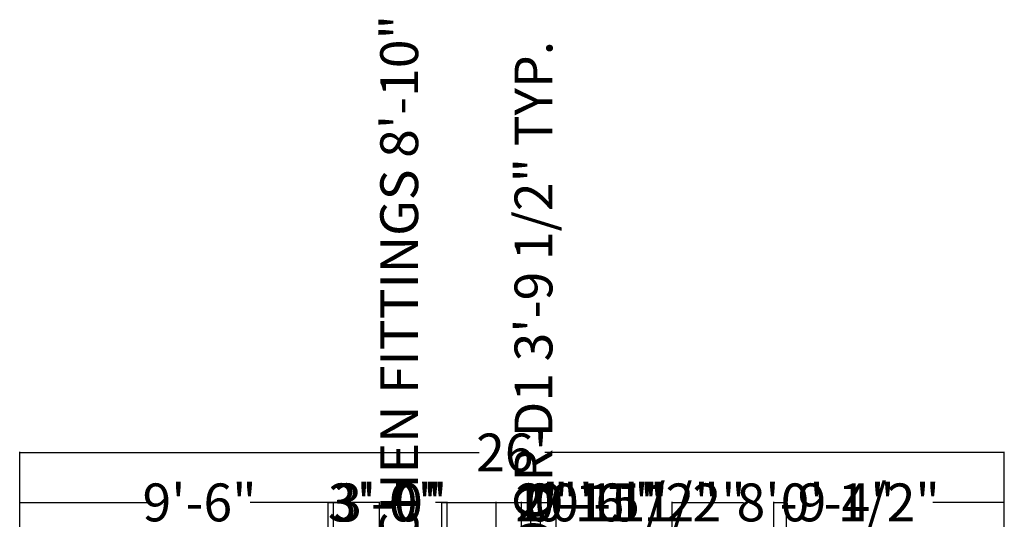
# Model space of a CAD drawing. Units: inches. Extents: x -51 to 1118, y -44 to 791.
# Tile 6 of 8: x 28 to 340, y 633 to 791. Entities that reach past the tile are written whole.
import ezdxf

# ---------------------------------------------------------------- set-up
doc = ezdxf.new("R2010")
doc.units = ezdxf.units.IN
doc.header["$MEASUREMENT"] = 0
doc.layers.add('A-ANNO-DIMS', color=2, linetype='Continuous', lineweight=18)
doc.styles.get("Standard").update_dxf_attribs({"font": 'arial.ttf'})
doc.dimstyles.get("Standard").update_dxf_attribs({"dimtxt": 12, "dimasz": 0.18, "dimexe": 0.18, "dimexo": 0.0625, "dimgap": 0.09, "dimtad": 0, "dimdec": 1, "dimzin": 0, "dimdsep": 46, "dimlunit": 3, "dimtxsty": 'Standard', "dimcen": 0.09, "dimadec": 0, "dimazin": 0, "dimtfac": 1, "dimtdec": 1, "dimtofl": 0, "dimtmove": 0, "dimatfit": 3, "dimfxl": 1, "dimtolj": 1, "dimtzin": 0, "dimarcsym": 0})

# ---------------------------------------------------------------- blocks, each defined once
blk = doc.blocks.new('*D10')
at = {"layer": 'A-ANNO-DIMS', "color": 0, "lineweight": -2, "transparency": 16777216}
for p, q in [((28.02, 606), (28.02, 654.38)), ((28.2, 654.2), (173.65, 654.2)), ((339.84, 654.2), (194.4, 654.2)), ((340.02, 606), (340.02, 654.38))]:
    blk.add_line(p, q, dxfattribs=at)
at = {"layer": 'A-ANNO-DIMS', "color": 0, "transparency": 16777216}
for points in [[(28.2, 654.23), (28.2, 654.17), (28.02, 654.2)], [(339.84, 654.23), (339.84, 654.17), (340.02, 654.2)]]:
    blk.add_solid(points, dxfattribs=at)
at = {"layer": 'Defpoints', "color": 0, "transparency": 16777216}
for p in [(340.02, 654.2), (28.02, 605.94), (340.02, 605.94)]:
    blk.add_point(p, dxfattribs=at)
at = {"layer": 'A-ANNO-DIMS', "color": 0, "transparency": 16777216, "insert": (184.02, 654.2), "char_height": 12, "attachment_point": 5}
blk.add_mtext("\\A1;26'", dxfattribs=at)
blk = doc.blocks.new('*D20')
at = {"layer": 'A-ANNO-DIMS', "color": 0, "lineweight": -2, "transparency": 16777216}
for p, q in [((184.08, 605.94), (191.01, 605.94)), ((190.83, 605.94), (190.83, 606.12)), ((190.83, 560.7), (190.83, 605.76)), ((184.08, 560.52), (191.01, 560.52))]:
    blk.add_line(p, q, dxfattribs=at)
at = {"layer": 'A-ANNO-DIMS', "color": 0, "transparency": 16777216}
for points in [[(190.8, 605.76), (190.86, 605.76), (190.83, 605.94)], [(190.8, 560.7), (190.86, 560.7), (190.83, 560.52)]]:
    blk.add_solid(points, dxfattribs=at)
at = {"layer": 'Defpoints', "color": 0, "transparency": 16777216}
for p in [(184.02, 605.94), (190.83, 605.94), (184.02, 560.52)]:
    blk.add_point(p, dxfattribs=at)
at = {"layer": 'A-ANNO-DIMS', "color": 0, "transparency": 16777216, "insert": (190.83, 696.98), "char_height": 12, "attachment_point": 5, "rotation": 90}
blk.add_mtext('\\A1;DOOR D1 3\'-9 1/2" TYP.', dxfattribs=at)
blk = doc.blocks.new('*D34')
at = {"layer": 'A-ANNO-DIMS', "color": 0, "lineweight": -2, "transparency": 16777216}
for p, q in [((132.45, 596.14), (148.46, 596.14)), ((148.28, 596.14), (148.28, 596.32)), ((148.28, 490.32), (148.28, 595.96)), ((132.45, 490.14), (148.46, 490.14))]:
    blk.add_line(p, q, dxfattribs=at)
at = {"layer": 'A-ANNO-DIMS', "color": 0, "transparency": 16777216}
for points in [[(148.25, 595.96), (148.31, 595.96), (148.28, 596.14)], [(148.25, 490.32), (148.31, 490.32), (148.28, 490.14)]]:
    blk.add_solid(points, dxfattribs=at)
at = {"layer": 'Defpoints', "color": 0, "transparency": 16777216}
for p in [(132.38, 596.14), (148.28, 596.14), (132.38, 490.14)]:
    blk.add_point(p, dxfattribs=at)
at = {"layer": 'A-ANNO-DIMS', "color": 0, "transparency": 16777216, "insert": (148.28, 696.39), "char_height": 12, "attachment_point": 5, "rotation": 90}
blk.add_mtext('\\A1;KITCHEN FITTINGS 8\'-10"', dxfattribs=at)
blk = doc.blocks.new('*D43')
at = {"layer": 'A-ANNO-DIMS', "color": 0, "lineweight": -2, "transparency": 16777216}
for p, q in [((187.02, 597), (187.02, 638.57)), ((187.2, 638.39), (192.84, 638.39)), ((193.02, 597), (193.02, 638.57)), ((193.02, 638.39), (193.2, 638.39))]:
    blk.add_line(p, q, dxfattribs=at)
at = {"layer": 'A-ANNO-DIMS', "color": 0, "transparency": 16777216}
for points in [[(187.2, 638.42), (187.2, 638.36), (187.02, 638.39)], [(192.84, 638.42), (192.84, 638.36), (193.02, 638.39)]]:
    blk.add_solid(points, dxfattribs=at)
at = {"layer": 'Defpoints', "color": 0, "transparency": 16777216}
for p in [(193.02, 638.39), (187.02, 596.94), (193.02, 596.94)]:
    blk.add_point(p, dxfattribs=at)
at = {"layer": 'A-ANNO-DIMS', "color": 0, "transparency": 16777216, "insert": (209.24, 638.39), "char_height": 12, "attachment_point": 5}
blk.add_mtext('\\A1;0\'-6"', dxfattribs=at)
blk = doc.blocks.new('*D48')
at = {"layer": 'A-ANNO-DIMS', "color": 0, "lineweight": -2, "transparency": 16777216}
for p, q in [((28.02, 606), (28.02, 638.57)), ((28.2, 638.39), (68.98, 638.39)), ((141.84, 638.39), (101.06, 638.39)), ((142.02, 606), (142.02, 638.57))]:
    blk.add_line(p, q, dxfattribs=at)
at = {"layer": 'A-ANNO-DIMS', "color": 0, "transparency": 16777216}
for points in [[(28.2, 638.42), (28.2, 638.36), (28.02, 638.39)], [(141.84, 638.42), (141.84, 638.36), (142.02, 638.39)]]:
    blk.add_solid(points, dxfattribs=at)
at = {"layer": 'Defpoints', "color": 0, "transparency": 16777216}
for p in [(142.02, 638.39), (28.02, 605.94), (142.02, 605.94)]:
    blk.add_point(p, dxfattribs=at)
at = {"layer": 'A-ANNO-DIMS', "color": 0, "transparency": 16777216, "insert": (85.02, 638.39), "char_height": 12, "attachment_point": 5}
blk.add_mtext('\\A1;9\'-6"', dxfattribs=at)
blk = doc.blocks.new('*D49')
at = {"layer": 'A-ANNO-DIMS', "color": 0, "lineweight": -2, "transparency": 16777216}
for p, q in [((234.77, 606), (234.77, 638.57)), ((234.95, 638.39), (257.37, 638.39)), ((339.84, 638.39), (317.42, 638.39)), ((340.02, 606), (340.02, 638.57))]:
    blk.add_line(p, q, dxfattribs=at)
at = {"layer": 'A-ANNO-DIMS', "color": 0, "transparency": 16777216}
for points in [[(234.95, 638.42), (234.95, 638.36), (234.77, 638.39)], [(339.84, 638.42), (339.84, 638.36), (340.02, 638.39)]]:
    blk.add_solid(points, dxfattribs=at)
at = {"layer": 'Defpoints', "color": 0, "transparency": 16777216}
for p in [(340.02, 638.39), (234.77, 605.94), (340.02, 605.94)]:
    blk.add_point(p, dxfattribs=at)
at = {"layer": 'A-ANNO-DIMS', "color": 0, "transparency": 16777216, "insert": (287.4, 638.39), "char_height": 12, "attachment_point": 5}
blk.add_mtext('\\A1;8\'-9 1/2"', dxfattribs=at)
blk = doc.blocks.new('*D55')
at = {"layer": 'A-ANNO-DIMS', "color": 0, "lineweight": -2, "transparency": 16777216}
for p, q in [((193.02, 108), (193.02, 638.57)), ((193.2, 638.39), (197.79, 638.39)), ((197.97, 108), (197.97, 638.57)), ((197.97, 638.39), (198.15, 638.39))]:
    blk.add_line(p, q, dxfattribs=at)
at = {"layer": 'A-ANNO-DIMS', "color": 0, "transparency": 16777216}
for points in [[(193.2, 638.42), (193.2, 638.36), (193.02, 638.39)], [(197.79, 638.42), (197.79, 638.36), (197.97, 638.39)]]:
    blk.add_solid(points, dxfattribs=at)
at = {"layer": 'Defpoints', "color": 0, "transparency": 16777216}
for p in [(197.97, 638.39), (193.02, 107.94), (197.97, 107.94)]:
    blk.add_point(p, dxfattribs=at)
at = {"layer": 'A-ANNO-DIMS', "color": 0, "transparency": 16777216, "insert": (214.19, 638.39), "char_height": 12, "attachment_point": 5}
blk.add_mtext('\\A1;0\'-5"', dxfattribs=at)
blk = doc.blocks.new('*D57')
at = {"layer": 'A-ANNO-DIMS', "color": 0, "lineweight": -2, "transparency": 16777216}
for p, q in [((179.02, 57), (179.02, 638.57)), ((179.2, 638.39), (189.84, 638.39)), ((190.02, 57), (190.02, 638.57)), ((190.02, 638.39), (190.2, 638.39))]:
    blk.add_line(p, q, dxfattribs=at)
at = {"layer": 'A-ANNO-DIMS', "color": 0, "transparency": 16777216}
for points in [[(179.2, 638.42), (179.2, 638.36), (179.02, 638.39)], [(189.84, 638.42), (189.84, 638.36), (190.02, 638.39)]]:
    blk.add_solid(points, dxfattribs=at)
at = {"layer": 'Defpoints', "color": 0, "transparency": 16777216}
for p in [(190.02, 638.39), (179.02, 56.94), (190.02, 56.94)]:
    blk.add_point(p, dxfattribs=at)
at = {"layer": 'A-ANNO-DIMS', "color": 0, "transparency": 16777216, "insert": (210.9, 638.39), "char_height": 12, "attachment_point": 5}
blk.add_mtext('\\A1;0\'-11"', dxfattribs=at)
blk = doc.blocks.new('*D61')
at = {"layer": 'A-ANNO-DIMS', "color": 0, "lineweight": -2, "transparency": 16777216}
for p, q in [((125.75, 324), (125.75, 638.57)), ((125.93, 638.39), (127.71, 638.39)), ((161.57, 638.39), (159.79, 638.39)), ((161.75, 324), (161.75, 638.57))]:
    blk.add_line(p, q, dxfattribs=at)
at = {"layer": 'A-ANNO-DIMS', "color": 0, "transparency": 16777216}
for points in [[(125.93, 638.42), (125.93, 638.36), (125.75, 638.39)], [(161.57, 638.42), (161.57, 638.36), (161.75, 638.39)]]:
    blk.add_solid(points, dxfattribs=at)
at = {"layer": 'Defpoints', "color": 0, "transparency": 16777216}
for p in [(161.75, 638.39), (125.75, 323.94), (161.75, 323.94)]:
    blk.add_point(p, dxfattribs=at)
at = {"layer": 'A-ANNO-DIMS', "color": 0, "transparency": 16777216, "insert": (143.75, 638.39), "char_height": 12, "attachment_point": 5}
blk.add_mtext('\\A1;3\'-0"', dxfattribs=at)
blk = doc.blocks.new('*D62')
at = {"layer": 'A-ANNO-DIMS', "color": 0, "lineweight": -2, "transparency": 16777216}
for p, q in [((161.75, 324), (161.75, 638.57)), ((161.93, 638.39), (186.84, 638.39)), ((187.02, 327), (187.02, 638.57)), ((187.02, 638.39), (187.2, 638.39))]:
    blk.add_line(p, q, dxfattribs=at)
at = {"layer": 'A-ANNO-DIMS', "color": 0, "transparency": 16777216}
for points in [[(161.93, 638.42), (161.93, 638.36), (161.75, 638.39)], [(186.84, 638.42), (186.84, 638.36), (187.02, 638.39)]]:
    blk.add_solid(points, dxfattribs=at)
at = {"layer": 'Defpoints', "color": 0, "transparency": 16777216}
for p in [(187.02, 638.39), (187.02, 326.94), (161.75, 323.94)]:
    blk.add_point(p, dxfattribs=at)
at = {"layer": 'A-ANNO-DIMS', "color": 0, "transparency": 16777216, "insert": (217.32, 638.39), "char_height": 12, "attachment_point": 5}
blk.add_mtext('\\A1;2\'-1 1/2"', dxfattribs=at)
blk = doc.blocks.new('*D63')
at = {"layer": 'A-ANNO-DIMS', "color": 0, "lineweight": -2, "transparency": 16777216}
for p, q in [((127.45, 453), (127.45, 638.57)), ((127.63, 638.39), (129.41, 638.39)), ((163.27, 638.39), (161.48, 638.39)), ((163.45, 453), (163.45, 638.57))]:
    blk.add_line(p, q, dxfattribs=at)
at = {"layer": 'A-ANNO-DIMS', "color": 0, "transparency": 16777216}
for points in [[(127.63, 638.42), (127.63, 638.36), (127.45, 638.39)], [(163.27, 638.42), (163.27, 638.36), (163.45, 638.39)]]:
    blk.add_solid(points, dxfattribs=at)
at = {"layer": 'Defpoints', "color": 0, "transparency": 16777216}
for p in [(163.45, 638.39), (127.45, 452.94), (163.45, 452.94)]:
    blk.add_point(p, dxfattribs=at)
at = {"layer": 'A-ANNO-DIMS', "color": 0, "transparency": 16777216, "insert": (145.45, 638.39), "char_height": 12, "attachment_point": 5}
blk.add_mtext('\\A1;3\'-0"', dxfattribs=at)
blk = doc.blocks.new('*D64')
at = {"layer": 'A-ANNO-DIMS', "color": 0, "lineweight": -2, "transparency": 16777216}
for p, q in [((163.45, 453), (163.45, 638.57)), ((163.63, 638.39), (186.84, 638.39)), ((187.02, 453), (187.02, 638.57)), ((187.02, 638.39), (187.2, 638.39))]:
    blk.add_line(p, q, dxfattribs=at)
at = {"layer": 'A-ANNO-DIMS', "color": 0, "transparency": 16777216}
for points in [[(163.63, 638.42), (163.63, 638.36), (163.45, 638.39)], [(186.84, 638.42), (186.84, 638.36), (187.02, 638.39)]]:
    blk.add_solid(points, dxfattribs=at)
at = {"layer": 'Defpoints', "color": 0, "transparency": 16777216}
for p in [(187.02, 638.39), (163.45, 452.94), (187.02, 452.94)]:
    blk.add_point(p, dxfattribs=at)
at = {"layer": 'A-ANNO-DIMS', "color": 0, "transparency": 16777216, "insert": (221.32, 638.39), "char_height": 12, "attachment_point": 5}
blk.add_mtext('\\A1;1\'-11 1/2"', dxfattribs=at)
blk = doc.blocks.new('*D65')
at = {"layer": 'A-ANNO-DIMS', "color": 0, "lineweight": -2, "transparency": 16777216}
for p, q in [((267.02, 366), (267.02, 638.57)), ((267.2, 638.39), (270.84, 638.39)), ((271.02, 366), (271.02, 638.57)), ((271.02, 638.39), (271.2, 638.39))]:
    blk.add_line(p, q, dxfattribs=at)
at = {"layer": 'A-ANNO-DIMS', "color": 0, "transparency": 16777216}
for points in [[(267.2, 638.42), (267.2, 638.36), (267.02, 638.39)], [(270.84, 638.42), (270.84, 638.36), (271.02, 638.39)]]:
    blk.add_solid(points, dxfattribs=at)
at = {"layer": 'Defpoints', "color": 0, "transparency": 16777216}
for p in [(271.02, 638.39), (267.02, 365.94), (271.02, 365.94)]:
    blk.add_point(p, dxfattribs=at)
at = {"layer": 'A-ANNO-DIMS', "color": 0, "transparency": 16777216, "insert": (287.24, 638.39), "char_height": 12, "attachment_point": 5}
blk.add_mtext('\\A1;0\'-4"', dxfattribs=at)

msp = doc.modelspace()

# ---------------------------------------------------------------- dimensions: what is measured, and where the dimension line sits
at = {"layer": 'A-ANNO-DIMS'}
for base, p1, p2, text, picture, middle in [((148.28, 596.14), (132.38, 490.14), (132.38, 596.14), 'KITCHEN FITTINGS <>', '*D34', (148.28, 696.39)), ((190.83, 605.94), (184.02, 560.52), (184.02, 605.94), 'DOOR D1 <> TYP.', '*D20', (190.83, 696.98))]:
    dim = msp.add_linear_dim(base=base, p1=p1, p2=p2, angle=90, text=text, dimstyle='Standard', override={"dimdec": 1, "dimlfac": 1, "dimrnd": 0, "dimzin": 1, "dimdsep": 46, "dimlunit": 4, "dimfrac": 2}, dxfattribs=at)
    dim.commit()
    dim.dimension.update_dxf_attribs({"geometry": picture, "text_midpoint": middle})
for base, p1, p2, override, picture, middle in [((340.02, 654.2), (28.02, 605.94), (340.02, 605.94), {"dimclrd": 0, "dimclre": 0, "dimclrt": 0}, '*D10', (184.02, 654.2)), ((187.02, 638.39), (161.75, 323.94), (187.02, 326.94), {"dimdec": 1, "dimlfac": 1, "dimrnd": 0, "dimzin": 1, "dimdsep": 46, "dimlunit": 4, "dimfrac": 2}, '*D62', (217.32, 638.39)), ((187.02, 638.39), (163.45, 452.94), (187.02, 452.94), {"dimdec": 1, "dimlfac": 1, "dimrnd": 0, "dimzin": 1, "dimdsep": 46, "dimlunit": 4, "dimfrac": 2}, '*D64', (221.32, 638.39)), ((340.0217, 638.3903), (234.7701, 605.9403), (340.0217, 605.9403), {"dimdec": 1, "dimlfac": 1, "dimrnd": 0, "dimzin": 1, "dimdsep": 46, "dimlunit": 4, "dimfrac": 2}, '*D49', (287.3959, 638.3903)), ((142.02, 638.39), (28.02, 605.94), (142.02, 605.94), {"dimdec": 1, "dimlfac": 1, "dimrnd": 0, "dimzin": 1, "dimdsep": 46, "dimlunit": 4, "dimfrac": 2}, '*D48', (85.02, 638.39)), ((161.75, 638.39), (125.75, 323.94), (161.75, 323.94), {"dimdec": 1, "dimlfac": 1, "dimrnd": 0, "dimzin": 1, "dimdsep": 46, "dimlunit": 4, "dimfrac": 2}, '*D61', (143.75, 638.39)), ((163.45, 638.39), (127.45, 452.94), (163.45, 452.94), {"dimdec": 1, "dimlfac": 1, "dimrnd": 0, "dimzin": 1, "dimdsep": 46, "dimlunit": 4, "dimfrac": 2}, '*D63', (145.45, 638.39)), ((190.02, 638.39), (179.02, 56.94), (190.02, 56.94), {"dimdec": 1, "dimlfac": 1, "dimrnd": 0, "dimzin": 1, "dimdsep": 46, "dimlunit": 4, "dimfrac": 2}, '*D57', (210.9, 638.39)), ((193.02, 638.39), (187.02, 596.94), (193.02, 596.94), {"dimdec": 1, "dimlfac": 1, "dimrnd": 0, "dimzin": 1, "dimdsep": 46, "dimlunit": 4, "dimfrac": 2}, '*D43', (209.24, 638.39)), ((197.9672, 638.3903), (193.0217, 107.9403), (197.9672, 107.9403), {"dimdec": 1, "dimlfac": 1, "dimrnd": 0, "dimzin": 1, "dimdsep": 46, "dimlunit": 4, "dimfrac": 2}, '*D55', (214.1868, 638.3903)), ((271.02, 638.39), (267.02, 365.94), (271.02, 365.94), {"dimdec": 1, "dimlfac": 1, "dimrnd": 0, "dimzin": 1, "dimdsep": 46, "dimlunit": 4, "dimfrac": 2}, '*D65', (287.24, 638.39))]:
    dim = msp.add_linear_dim(base=base, p1=p1, p2=p2, dimstyle='Standard', override=override, dxfattribs=at)
    dim.commit()
    dim.dimension.update_dxf_attribs({"geometry": picture, "text_midpoint": middle})

doc.saveas('drawing.dxf')
